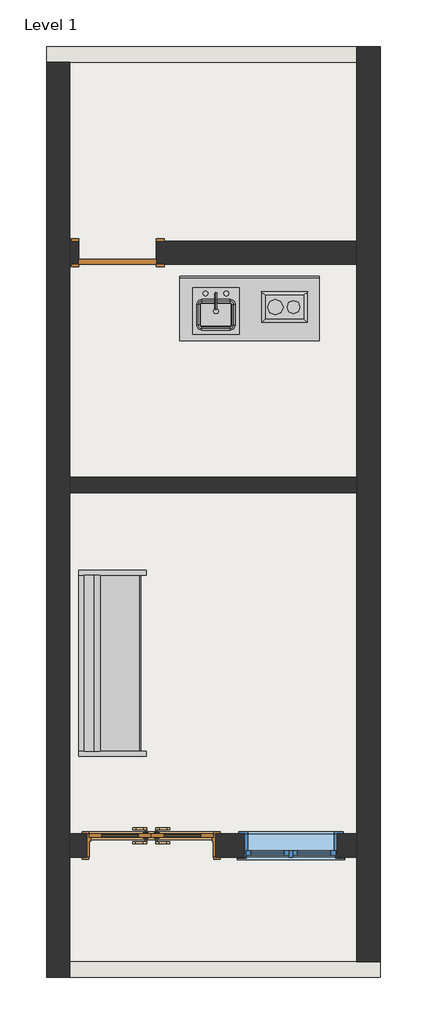
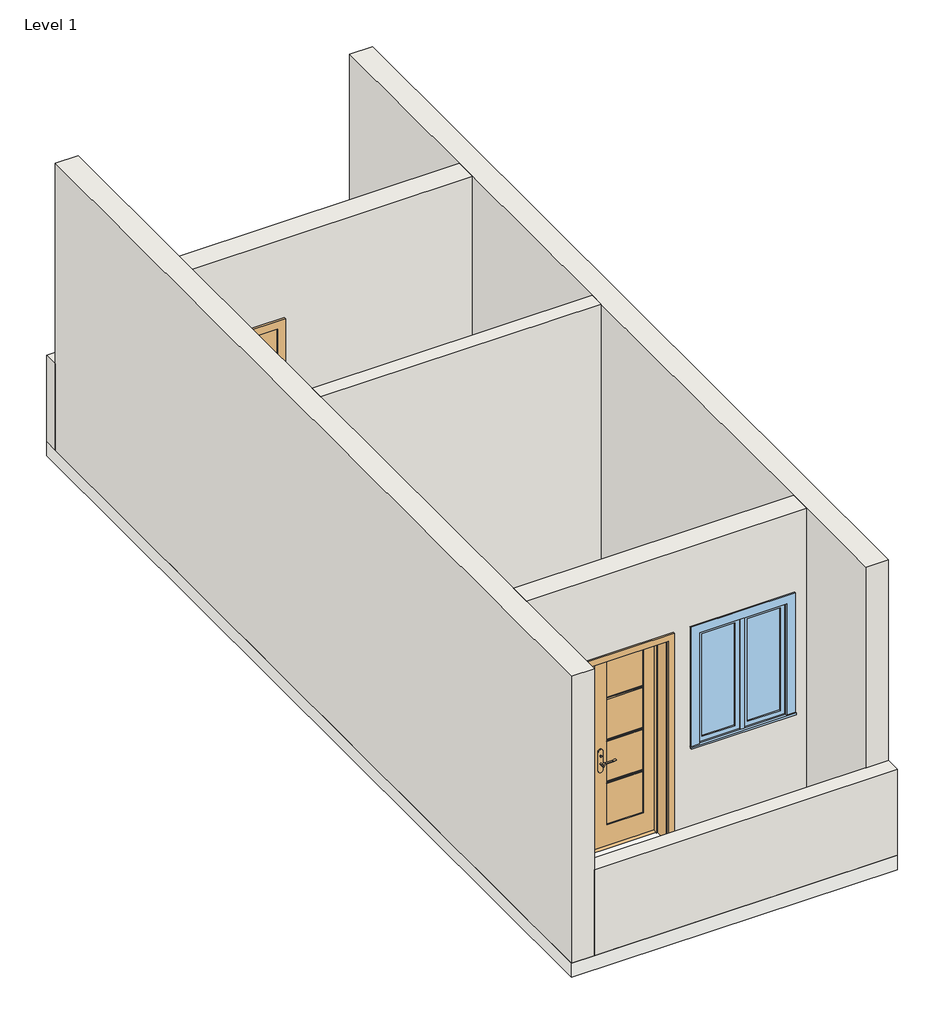
# One storey: 7 walls, 2 doors, 2 furniture elements, 2 proxies, 1 flow terminal, 1 slab, 1 window.
"""IFC4 building model written with IfcOpenShell, lengths in millimetres."""

from ifc_helpers import new_model, si_unit, frame, origin, origin_with_axes, place, context, project, spatial, polyline, outline, extrude, faceted_brep, transform, mapped, element, save
from components import proxy_fe84b772, proxy_844211aa, door_4500b467, single_flush_2_5_bb98abfd, flow_terminal_871c2e40, furniture_b3f308bd, furniture_a4ffab56, window_419b5846

model = new_model("IFC4")

# Units and contexts
model_context = context("Model", 3, world=origin())
ifc_project = project(units=[si_unit("LENGTHUNIT", "METRE", prefix="MILLI")], contexts=[model_context])

# Site, building, storey
site = spatial("IfcSite", under=ifc_project)
building = spatial("IfcBuilding", under=site)
storey = spatial("IfcBuildingStorey", under=building, Name="Level 1", Elevation=0.0)

# Proxies
placement = place(None, origin())
proxy_shape = proxy_fe84b772(model_context)
element("IfcBuildingElementProxy", 1, Name="Cook Top-2 Unit : 12\" x 18\"", ObjectType="Cook Top-2 Unit : 12\" x 18\"", at=placement, inside=storey, context=model_context, shape_type="MappedRepresentation", body=[
    mapped(proxy_shape, transform((-4554.1941125, 4213.6297066, 0.0), x_axis=(0.0, 1.0, 0.0), y_axis=(-1.0, 0.0, 0.0), z_axis=(0.0, 0.0, 1.0))),
])
proxy_2_shape = proxy_844211aa(model_context)
element("IfcBuildingElementProxy", 2, Name="Kitchenette - Small : 54\"", ObjectType="Kitchenette - Small : 54\"", at=placement, inside=storey, context=model_context, shape_type="MappedRepresentation", body=[
    mapped(proxy_2_shape, transform((-4946.056613, 4594.6297066, 0.0), x_axis=(1.0, 0.0, 0.0), y_axis=(0.0, 1.0, 0.0), z_axis=(0.0, 0.0, 1.0))),
])

# Doors
door_shape = door_4500b467(model_context)
element("IfcDoor", 3, ObjectType="Door-Exterior-Double-Full Glass-Wood_Clad : 48\" x 84\"", at=placement, inside=storey, context=model_context, shape_type="MappedRepresentation", body=[
    mapped(door_shape, transform((-5892.5189081, -996.5452934, 0.0), x_axis=(1.0, 0.0, 0.0), y_axis=(0.0, 1.0, 0.0), z_axis=(0.0, 0.0, 1.0))),
])
single_flush_2_5_shape = single_flush_2_5_bb98abfd(model_context)
element("IfcDoor", 4, ObjectType="Single-Flush : 2.5'", at=placement, inside=storey, context=model_context, shape_type="MappedRepresentation", body=[
    mapped(single_flush_2_5_shape, transform((-6222.7189081, 4823.2297066, 0.0), x_axis=(-1.0, 0.0, 0.0), y_axis=(0.0, -1.0, 0.0), z_axis=(0.0, 0.0, 1.0))),
])

# Flow terminal
flow_terminal_shape = flow_terminal_871c2e40(model_context)
element("IfcFlowTerminal", 5, ObjectType="Sink Kitchen-Island : 18\" x 18\"", at=placement, inside=storey, context=model_context, shape_type="MappedRepresentation", body=[
    mapped(flow_terminal_shape, transform((-5273.2081486, 4249.3843055, 0.0), x_axis=(1.0, 0.0, 0.0), y_axis=(0.0, 1.0, 0.0), z_axis=(0.0, 0.0, 1.0))),
])

# Furniture
furniture_shape = furniture_b3f308bd(model_context)
element("IfcFurniture", 6, ObjectType="Counter Top w Sink Hole : 24\" Depth", at=placement, inside=storey, context=model_context, shape_type="MappedRepresentation", body=[
    mapped(furniture_shape, transform((-4412.656613, 4594.6297066, 0.0), x_axis=(1.0, 0.0, 0.0), y_axis=(0.0, 1.0, 0.0), z_axis=(0.0, 0.0, 1.0))),
])
furniture_2_shape = furniture_a4ffab56(model_context)
element("IfcFurniture", 7, ObjectType="Sofa : 72\"", at=placement, inside=storey, context=model_context, shape_type="MappedRepresentation", body=[
    mapped(furniture_2_shape, transform((-6127.3648097, 720.6092148, 0.0), x_axis=(0.0, 1.0000000000000002, 0.0), y_axis=(-1.0000000000000002, 0.0, 0.0), z_axis=(0.0, 0.0, 1.0))),
])

# Slab
element("IfcSlab", 8, ObjectType="6\"", at=placement, inside=storey, context=model_context, shape_type="SweptSolid", body=[
    extrude(outline(polyline([(-3644.6189081, 6848.8797066), (-3644.6189081, -2295.1202934), (-6921.2189081, -2295.1202934), (-6921.2189081, 6848.8797066), (-3644.6189081, 6848.8797066)])), frame((0.0, 0.0, -152.4), z_axis=(0.0, 0.0, 1.0), x_axis=(1.0, 0.0, 0.0)), (0.0, 0.0, 1.0), 152.4),
])

# Walls
element("IfcWall", 9, ObjectType="6\"", at=placement, inside=storey, context=model_context, shape_type="Brep", body=[
    faceted_brep([(-6921.2189081, 6696.4797066, 0.0), (-6692.6189081, 6696.4797066, 0.0), (-3873.2189081, 6696.4797066, 0.0), (-3873.2189081, 6696.4797066, 914.4), (-6921.2189081, 6696.4797066, 914.4), (-6921.2189081, 6848.8797066, 0.0), (-6921.2189081, 6848.8797066, 914.4), (-3873.2189081, 6848.8797066, 914.4), (-3873.2189081, 6848.8797066, 0.0)], [[[0, 1, 2, 3, 4]], [[5, 6, 7, 8]], [[2, 1, 0, 5, 8]], [[4, 3, 7, 6]], [[0, 4, 6, 5]], [[3, 2, 8, 7]]]),
])
element("IfcWall", 10, ObjectType="6\"", at=placement, inside=storey, context=model_context, shape_type="Brep", body=[
    faceted_brep([(-3644.6189081, -2142.7202934, 0.0), (-3873.2189081, -2142.7202934, 0.0), (-6692.6189081, -2142.7202934, 0.0), (-6692.6189081, -2142.7202934, 914.4), (-3644.6189081, -2142.7202934, 914.4), (-3644.6189081, -2295.1202934, 0.0), (-3644.6189081, -2295.1202934, 914.4), (-6692.6189081, -2295.1202934, 914.4), (-6692.6189081, -2295.1202934, 0.0)], [[[0, 1, 2, 3, 4]], [[5, 6, 7, 8]], [[2, 1, 0, 5, 8]], [[4, 3, 7, 6]], [[0, 4, 6, 5]], [[3, 2, 8, 7]]]),
])
element("IfcWall", 11, ObjectType="6\"", at=placement, inside=storey, context=model_context, shape_type="SweptSolid", body=[
    extrude(outline(polyline([(-6692.6189081, 2619.7797066), (-3873.2189081, 2619.7797066), (-3873.2189081, 2467.3797066), (-6692.6189081, 2467.3797066), (-6692.6189081, 2619.7797066)])), origin_with_axes(), (0.0, 0.0, 1.0), 3048.0),
])
element("IfcWall", 12, ObjectType="9\"", at=placement, inside=storey, context=model_context, shape_type="Brep", body=[
    faceted_brep([(-6692.6189081, -2295.1202934, 0.0), (-6692.6189081, -2142.7202934, 0.0), (-6692.6189081, -1114.0202934, 0.0), (-6692.6189081, -885.4202934, 0.0), (-6692.6189081, 2467.3797066, 0.0), (-6692.6189081, 2619.7797066, 0.0), (-6692.6189081, 4708.9297066, 0.0), (-6692.6189081, 4937.5297066, 0.0), (-6692.6189081, 6696.4797066, 0.0), (-6692.6189081, 6696.4797066, 3048.0), (-6692.6189081, 4937.5297066, 3048.0), (-6692.6189081, 4708.9297066, 3048.0), (-6692.6189081, 2619.7797066, 3048.0), (-6692.6189081, 2467.3797066, 3048.0), (-6692.6189081, -885.4202934, 3048.0), (-6692.6189081, -1114.0202934, 3048.0), (-6692.6189081, -2295.1202934, 3048.0), (-6692.6189081, -2295.1202934, 914.4), (-6921.2189081, -2295.1202934, 0.0), (-6921.2189081, -2295.1202934, 3048.0), (-6921.2189081, 6696.4797066, 3048.0), (-6921.2189081, 6696.4797066, 914.4), (-6921.2189081, 6696.4797066, 0.0)], [[[0, 1, 2, 3, 4, 5, 6, 7, 8, 9, 10, 11, 12, 13, 14, 15, 16, 17]], [[18, 19, 20, 21, 22]], [[8, 7, 6, 5, 4, 3, 2, 1, 0, 18, 22]], [[16, 15, 14, 13, 12, 11, 10, 9, 20, 19]], [[0, 17, 16, 19, 18]], [[9, 8, 22, 21, 20]]]),
])
element("IfcWall", 13, ObjectType="9\"", at=placement, inside=storey, context=model_context, shape_type="Brep", body=[
    faceted_brep([(-3873.2189081, 6848.8797066, 0.0), (-3873.2189081, 6696.4797066, 0.0), (-3873.2189081, 4937.5297066, 0.0), (-3873.2189081, 4708.9297066, 0.0), (-3873.2189081, 2619.7797066, 0.0), (-3873.2189081, 2467.3797066, 0.0), (-3873.2189081, -885.4202934, 0.0), (-3873.2189081, -1114.0202934, 0.0), (-3873.2189081, -2142.7202934, 0.0), (-3873.2189081, -2142.7202934, 3048.0), (-3873.2189081, -1114.0202934, 3048.0), (-3873.2189081, -885.4202934, 3048.0), (-3873.2189081, 2467.3797066, 3048.0), (-3873.2189081, 2619.7797066, 3048.0), (-3873.2189081, 4708.9297066, 3048.0), (-3873.2189081, 4937.5297066, 3048.0), (-3873.2189081, 6848.8797066, 3048.0), (-3873.2189081, 6848.8797066, 914.4), (-3644.6189081, 6848.8797066, 0.0), (-3644.6189081, 6848.8797066, 3048.0), (-3644.6189081, -2142.7202934, 3048.0), (-3644.6189081, -2142.7202934, 914.4), (-3644.6189081, -2142.7202934, 0.0)], [[[0, 1, 2, 3, 4, 5, 6, 7, 8, 9, 10, 11, 12, 13, 14, 15, 16, 17]], [[18, 19, 20, 21, 22]], [[8, 7, 6, 5, 4, 3, 2, 1, 0, 18, 22]], [[16, 15, 14, 13, 12, 11, 10, 9, 20, 19]], [[0, 17, 16, 19, 18]], [[9, 8, 22, 21, 20]]]),
])
element("IfcWall", 14, ObjectType="9\"", at=placement, inside=storey, context=model_context, shape_type="SweptSolid", body=[
    extrude(outline(polyline([(3048.0, -3873.2189081), (3048.0, -6692.6189081), (0.0, -6692.6189081), (0.0, -6527.5189081), (2159.0, -6527.5189081), (2159.0, -5257.5189081), (0.0, -5257.5189081), (0.0, -3873.2189081), (3048.0, -3873.2189081)]), holes=[polyline([(2133.6, -4978.1189081), (2133.6, -4063.7189081), (914.4, -4063.7189081), (914.4, -4978.1189081), (2133.6, -4978.1189081)])]), frame((0.0, -1114.0202934, 0.0), z_axis=(0.0, 1.0, 0.0), x_axis=(0.0, 0.0, 1.0)), (0.0, 0.0, 1.0), 228.6),
])
element("IfcWall", 15, ObjectType="9\"", at=placement, inside=storey, context=model_context, shape_type="SweptSolid", body=[
    extrude(outline(polyline([(0.0, -6692.6189081), (0.0, -6603.7189081), (2133.6, -6603.7189081), (2133.6, -5841.7189081), (0.0, -5841.7189081), (0.0, -3873.2189081), (3048.0, -3873.2189081), (3048.0, -6692.6189081), (0.0, -6692.6189081)])), frame((0.0, 4708.9297066, 0.0), z_axis=(0.0, 1.0, 0.0), x_axis=(0.0, 0.0, 1.0)), (0.0, 0.0, 1.0), 228.6),
])

# Window
window_shape = window_419b5846(model_context)
element("IfcWindow", 16, ObjectType="Casement Dbl with Trim : 36\" x 48\"", at=placement, inside=storey, context=model_context, shape_type="MappedRepresentation", body=[
    mapped(window_shape, transform((-4520.9189081, -980.6702934, 0.0), x_axis=(-1.0, 0.0, 0.0), y_axis=(0.0, -1.0, 0.0), z_axis=(0.0, 0.0, 1.0))),
])

save(model, "model.ifc")

# Revit data of these elements
# Type "Cook Top-2 Unit : 12\" x 18\""
#   Assembly Code = "E1090400"
#   Counter Height = 3' - 0"
#   Depth = 1' - 6"
#   Width = 1' - 0"
#   Burner Material = Steel, Chrome Plated
#   Cooktop Material = Steel, Polished
#   Default Elevation = 0
# Type "Kitchenette - Small : 54\""
#   Assembly Code = "E1090400"
#   Width = 4' - 6"
#   Height = 2' - 10 1/2"
#   Depth = 2' - 0"
#   Toe Depth = 0' - 3"
#   Toe Height = 0' - 3 1/2"
#   Cabinet Material = Cabinets
#   Door/Drawer Material = Cabinets
#   Handle Material = Cabinets - Handles
#   Default Elevation = 0
# Type "Door-Exterior-Double-Full Glass-Wood_Clad : 48\" x 84\""
#   Type Mark = "9"
#   Assembly Code = "B2030100"
#   Analytic Construction = "French door, wood frame with double glass"
#   Top Rail = 0' - 4 11/16"
#   Threshold Offset [instance default] = 0' - 0 1/2"
#   Thickness = 0' - 1 3/8"
#   Thermal Resistance (R) = 1.9158 (h·ft²·°F)/BTU
#   Swing Angle [instance default] = 90.00°
#   Stiles = 0' - 4 3/4"
#   Rough Width = 4' - 2"
#   Rough Height = 7' - 1"
#   Panel Width = 2' - 0"
#   Door Offset [instance default] = 0' - 0"
#   Height = 7' - 0"
#   Width = 4' - 0"
#   Heat Transfer Coefficient (U) = 0.5220 BTU/(h·ft²·°F)
#   Bottom Rail = 0' - 9 1/8"
#   Exterior Trim [instance default] = yes
#   Threshold [instance default] = yes
#   Show Grill [instance default] = yes
#   Function = 1
#   Trim Material = Cherry
#   Threshold Material = Cherry
#   Panel Material = Cherry
#   Glazing = Glass
#   Frame Material = Cherry
#   Door Handle Material = Aluminum
#   Visual Light Transmittance = 0
#   Solar Heat Gain Coefficient = 0
#   Wall Closure = (empty or 0)
#   Construction Type = (empty or 0)
# Type "Single-Flush : 2.5'"
#   Type Mark = "8"
#   Construction Type Id = "MDOOR"
#   Assembly Code = "C1020"
#   Analytic Construction = "Metal"
#   Thickness = 0' - 2"
#   Heat Transfer Coefficient (U) = 0.651978 BTU/(h·ft²·°F)
#   Height = 7' - 0"
#   Trim Projection Ext = 0' - 1"
#   Trim Projection Int = 0' - 1"
#   Trim Width = 0' - 3"
#   Width = 2' - 6"
#   Define Thermal Properties by = 1
#   Door Material = Door - Panel
#   Frame Material = Door - Frame
#   Visual Light Transmittance = 0
#   Solar Heat Gain Coefficient = 0
#   Function = (empty or 0)
#   Wall Closure = (empty or 0)
# Type "Sink Kitchen-Island : 18\" x 18\""
#   Assembly Code = "D2010410"
#   Counter Height = 3' - 0"
#   Depth = 1' - 6"
#   Width = 1' - 6"
#   Faucet Material = Steel, Polished
#   Sink Material = Steel, Polished
#   Default Elevation = 0
# Type "Counter Top w Sink Hole : 24\" Depth"
#   Assembly Code = "C1030400"
#   Counter Thickness = 0' - 1 1/2"
#   Depth = 2' - 1"
#   Height = 3' - 0"
#   Length [instance default] = 8' - 0"
#   Sink Location [instance default] = 2' - 0"
#   Sink Location To Wall [instance default] = 0' - 6"
#   Sink Opening Depth [instance default] = 1' - 3"
#   Sink Opening Width [instance default] = 2' - 3"
#   Counter Top Material = none
#   Default Elevation = 0
# Type "Sofa : 72\""
#   Assembly Code = "E2020200"
#   Width = 6' - 0"
#   Seat Material = Linen, Beige
#   Frame Material = Cherry
#   Default Elevation = 0
# Type "6\""
#   Assembly Code = "B1010"
#   Function = 0
#   Layers, outside or top first: 0' - 6" no material (function 1)
# Type "6\""
#   Assembly Code = "B2010"
#   Layers, outside or top first: 0' - 6" no material (function 1)
# Type "9\""
#   Assembly Code = "B2010"
#   Layers, outside or top first: 0' - 9" no material (function 1)
# Type "Casement Dbl with Trim : 36\" x 48\""
#   Type Mark = "19"
#   Construction Type Id = "GSP4R"
#   Assembly Code = "B2020100"
#   Analytic Construction = "1/8 in Pilkington single glazing"
#   Visual Light Transmittance = 0.9
#   Solar Heat Gain Coefficient = 0.78
#   Heat Transfer Coefficient (U) = 0.6496 BTU/(h·ft²·°F)
#   Height = 4' - 0"
#   Default Sill Height = 3' - 0"
#   Trim Projection - Ext. = 0' - 0 1/2"
#   Trim Projection - Int. = 0' - 0 3/4"
#   Trim Width - Exterior = 0' - 3 1/2"
#   Trim Width - Interior = 0' - 3 1/2"
#   Width = 3' - 0"
#   Window Inset = 0' - 0 3/4"
#   Define Thermal Properties by = 1
#   Glass Pane Material = Glass
#   Sash Material = Sash
#   Trim Exterior Material = Trim
#   Trim Interior Material = Trim
#   Wall Closure = (empty or 0)
# Element 1 (IfcBuildingElementProxy, "Cook Top-2 Unit : 12\" x 18\"")
#   Phase Created = New Construction
#   Materials on its faces: "Steel, Chrome Plated", "Steel, Polished"
# Element 2 (IfcBuildingElementProxy, "Kitchenette - Small : 54\"")
#   Phase Created = New Construction
#   Materials on its faces: "Cabinets", "Cabinets - Handles"
# Element 3 (IfcDoor, "Door-Exterior-Double-Full Glass-Wood_Clad : 48\" x 84\"")
#   Threshold Offset = 0' - 0 1/2"
#   Swing Angle = 90.00°
#   Door Offset = 0' - 0"
#   Threshold = yes
#   Show Grill = yes
#   Exterior Trim = yes
#   Phase Created = New Construction
#   Materials on its faces: "Cherry", "Aluminum", "Glass"
# Element 4 (IfcDoor, "Single-Flush : 2.5'")
#   Phase Created = New Construction
#   Materials on its faces: "Door - Frame", "Door - Panel"
# Element 5 (IfcFlowTerminal, "Sink Kitchen-Island : 18\" x 18\"")
#   Mark = "2"
#   Phase Created = New Construction
#   Materials on its faces: "Steel, Polished"
# Element 6 (IfcFurniture, "Counter Top w Sink Hole : 24\" Depth")
#   Sink Opening Depth = 1' - 3"
#   Sink Location To Wall = 0' - 6"
#   Length = 4' - 6"
#   Sink Location = 1' - 2"
#   Sink Opening Width = 1' - 4"
#   Phase Created = New Construction
#   Materials on its faces: "Counter Top"
# Element 7 (IfcFurniture, "Sofa : 72\"")
#   Phase Created = New Construction
#   Materials on its faces: "Cherry", "Linen, Beige"
# Element 8 (IfcSlab, "6\"")
#   Height Offset From Level = 0' - 0"
#   Phase Created = New Construction
#   Materials on its faces: "Default Floor"
# Elements 9, 10 (IfcWall, "6\"")
#   Top Offset = 0' - 0"
#   Base Offset = 0' - 0"
#   Unconnected Height = 3' - 0"
#   wall height = 3' - 0"
#   Phase Created = New Construction
#   Base Constraint = Level 1
#   Materials on its faces: "Default Wall"
# Element 11 (IfcWall, "6\"")
#   Top Offset = 0' - 0"
#   Base Offset = 0' - 0"
#   Unconnected Height = 10' - 0"
#   wall height = 10' - 0"
#   Phase Created = New Construction
#   Base Constraint = Level 1
#   Materials on its faces: "Default Wall"
# Elements 12, 13, 14, 15 (IfcWall, "9\"")
#   Top Offset = 0' - 0"
#   Base Offset = 0' - 0"
#   Unconnected Height = 10' - 0"
#   wall height = 10' - 0"
#   Phase Created = New Construction
#   Base Constraint = Level 1
#   Materials on its faces: "Default Wall"
# Element 16 (IfcWindow, "Casement Dbl with Trim : 36\" x 48\"")
#   Mark = "2"
#   Phase Created = New Construction
#   Materials on its faces: "Sash", "Trim", "Glass"
# Materials
#   "Steel, Chrome Plated": class "Metal", colour RGB 17 17 17, transparency 0, Description = "Chromiuim plated steel", Cost = 0
#   "Steel, Polished": class "Metal", colour RGB 57 57 57, transparency 0, Description = "Polished steel", Cost = 0
#   "Cabinets": colour RGB 249 249 249, transparency 0
#   "Cabinets - Handles": class "Metal", colour RGB 57 57 57, transparency 0
#   "Cherry": class "Wood", colour RGB 226 177 128, transparency 0, Description = "Prunus Serotina", Cost = 0
#   "Glass": class "Glass", colour RGB 0 128 192, transparency 0.75, Description = "Soda Lime Glass", Cost = 0
#   "Aluminum": class "Metal", colour RGB 247 247 247, transparency 0, Description = "Aluminum 6061", Cost = 0
#   "Door - Panel": class "Wood", colour RGB 210 159 95, transparency 0
#   "Door - Frame": colour RGB 118 70 51, transparency 0
#   "Linen, Beige": class "Textile", colour RGB 249 239 230, transparency 0, Description = "Linen, beige", Cost = 0
#   "Sash": class "Wood", colour RGB 224 178 126, transparency 0
#   "Trim": class "Wood", colour RGB 224 178 126, transparency 0
#   "Counter Top": class "Wood", colour RGB 226 177 128, transparency 0
#   "Default Floor": colour RGB 128 128 128, transparency 0
#   "Default Wall": colour RGB 128 128 128, transparency 0
